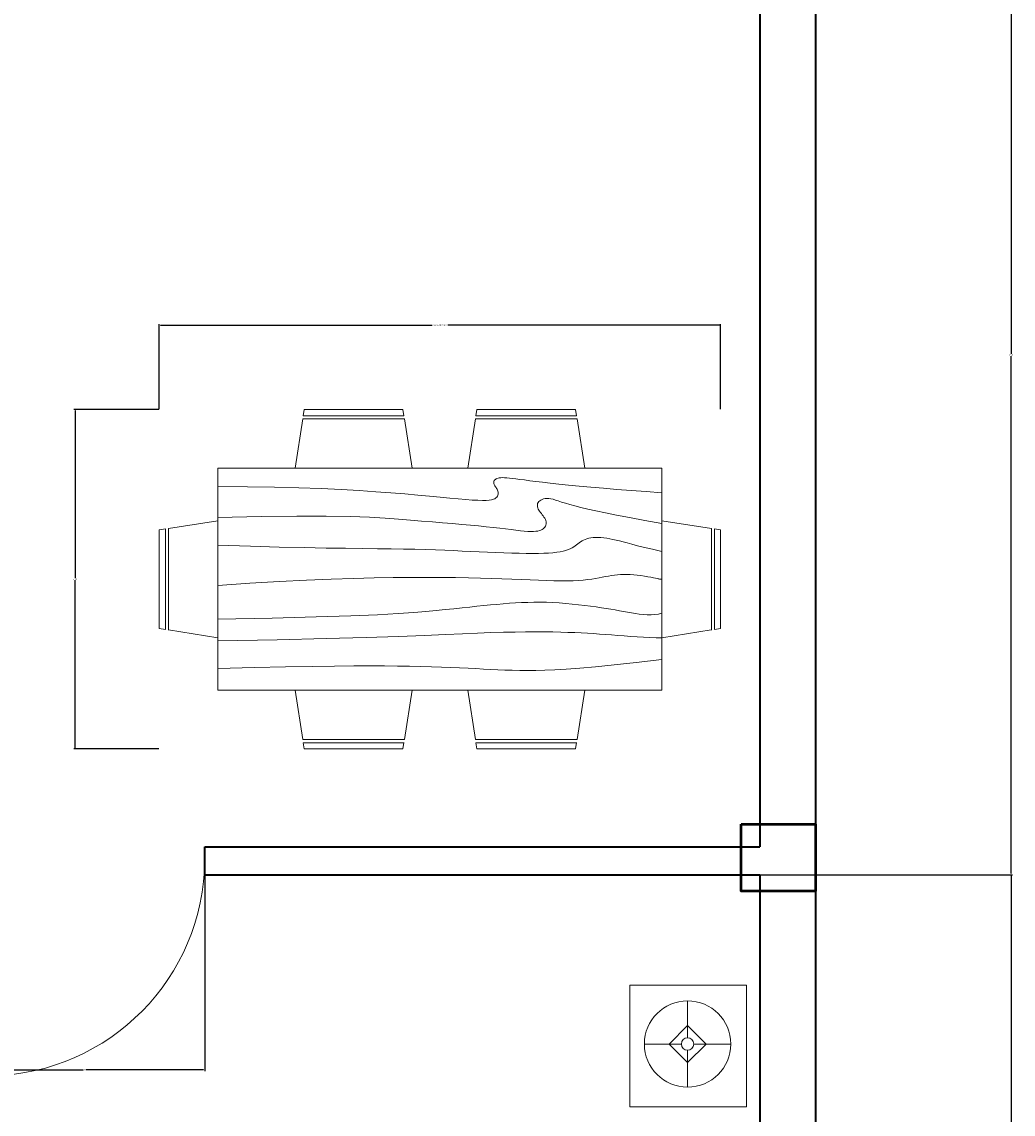
# Model space of a CAD drawing. Units: inches. Extents: x 50 to 2003, y -28 to 675.
# Tile 7 of 10: x 795 to 956, y 160 to 337. Entities that reach past the tile are written whole.
import ezdxf

# ---------------------------------------------------------------- set-up
doc = ezdxf.new("R2010")
doc.units = ezdxf.units.IN
for name, color, linetype, lineweight in [('A-ANNO-DIMS', 2, 'Continuous', 18), ('A-COLS', 1, 'Continuous', 50), ('A-DOOR', 4, 'Continuous', 18), ('A-FURN', 8, 'Continuous', 18), ('A-FURN-LITE', 9, 'Continuous', 13), ('A-WALL', 7, 'Continuous', 35)]:
    doc.layers.add(name, color=color, linetype=linetype, lineweight=lineweight)
doc.styles.get("Standard").update_dxf_attribs({"font": 'arial.ttf'})
doc.dimstyles.get("Standard").update_dxf_attribs({"dimtxt": 0.18, "dimasz": 0.18, "dimexe": 0.18, "dimexo": 0.0625, "dimgap": 0.09, "dimtad": 0, "dimtih": 1, "dimtoh": 1, "dimdec": 4, "dimzin": 0, "dimdsep": 46, "dimtxsty": 'Standard', "dimcen": 0.09, "dimadec": 0, "dimazin": 0, "dimtfac": 1, "dimtdec": 4, "dimtofl": 0, "dimtmove": 0, "dimatfit": 3, "dimfxl": 1, "dimtolj": 1, "dimtzin": 0, "dimarcsym": 0})

# ---------------------------------------------------------------- blocks, each defined once
blk = doc.blocks.new('Dining Set - 36 x 72 in.')
for p, q in [((-22, 27.5), (-22.1562, 26.50042)), ((-22, 27.5), (-6, 27.5)), ((-5.8437, 26.49966), (-6, 27.5)), ((6, 27.5), (5.8438, 26.50042)), ((6, 27.5), (22, 27.5)), ((22.1563, 26.49966), (22, 27.5)), ((-22.2343, 26.00059), (-23.4847, 17.99762)), ((-22.2304, 26), (-5.7608, 26)), ((-5.8416, 26.5), (-22.1534, 26.5)), ((-4.5152, 17.99762), (-5.7655, 25.99926)), ((5.7657, 26.00059), (4.5153, 17.99762)), ((5.7696, 26), (22.2392, 26)), ((22.1584, 26.5), (5.8466, 26.5)), ((23.4848, 17.99762), (22.2345, 25.99926)), ((36, 18), (-36, 18)), ((-36, 18), (-36, -18)), ((36, -18), (36, 18)), ((-44.0006, 8.23428), (-35.9976, 9.48474)), ((44.0006, 8.23428), (35.9976, 9.48474)), ((-45.5, 8), (-44.5004, 8.15617)), ((-45.5, 8), (-45.5, -8)), ((-44.5, -8.15843), (-44.5, 8.15338)), ((-44, 8.23041), (-44, -8.23915)), ((44, 8.23041), (44, -8.23915)), ((44.5, -8.15843), (44.5, 8.15338)), ((45.5, 8), (44.5005, 8.15617)), ((45.5, 8), (45.5, -8)), ((-44.4997, -8.15631), (-45.5, -8)), ((-35.9976, -9.48476), (-43.9993, -8.2345)), ((35.9976, -9.48476), (43.9993, -8.2345)), ((44.4997, -8.15631), (45.5, -8)), ((-36, -18), (36, -18)), ((-22.2343, -26.0006), (-23.4847, -17.99762)), ((-4.5152, -17.99762), (-5.7655, -25.99928)), ((5.7657, -26.0006), (4.5153, -17.99762)), ((23.4848, -17.99762), (22.2345, -25.99928)), ((-22.2304, -26), (-5.7608, -26)), ((-22, -27.5), (-22.1562, -26.50044)), ((-5.8416, -26.5), (-22.1534, -26.5)), ((-5.8437, -26.49967), (-6, -27.5)), ((5.7696, -26), (22.2392, -26)), ((6, -27.5), (5.8438, -26.50044)), ((22.1584, -26.5), (5.8466, -26.5)), ((22.1563, -26.49967), (22, -27.5)), ((-22, -27.5), (-6, -27.5)), ((6, -27.5), (22, -27.5))]:
    blk.add_line(p, q)
for points in [[(-36, 15), (-31.1772, 14.97754), (-26.8079, 14.91406), (-22.8538, 14.81543), (-19.276, 14.6875), (-16.0362, 14.53613), (-13.0957, 14.36718), (-10.4159, 14.18652), (-7.9583, 14), (-5.6904, 13.81315), (-3.6035, 13.63021), (-1.6954, 13.45508), (0.0365, 13.29166), (1.5945, 13.14388), (2.9811, 13.01562), (4.1988, 12.9108), (5.25, 12.83333), (6.1393, 12.78613), (6.8802, 12.76823), (7.4883, 12.77767), (7.9792, 12.8125), (8.3685, 12.87077), (8.6719, 12.95052), (8.9049, 13.0498), (9.0833, 13.16666), (9.2205, 13.29899), (9.3216, 13.44401), (9.3895, 13.59879), (9.4271, 13.76041), (9.4373, 13.92594), (9.4232, 14.09245), (9.3875, 14.257), (9.3333, 14.41666), (9.2638, 14.56917), (9.1836, 14.71484), (9.0975, 14.85465), (9.0104, 14.98958), (8.9272, 15.1206), (8.8529, 15.2487), (8.7922, 15.37483), (8.75, 15.5), (8.7305, 15.62467), (8.7344, 15.74739), (8.7617, 15.86621), (8.8125, 15.97916), (8.8867, 16.08431), (8.9844, 16.17968), (9.1055, 16.26334), (9.25, 16.33333), (9.4189, 16.38802), (9.6172, 16.42708), (9.8506, 16.45052), (10.125, 16.45833), (10.4463, 16.45052), (10.8203, 16.42708), (11.2529, 16.38802), (11.75, 16.33333), (12.3184, 16.26318), (12.9694, 16.17838), (13.7151, 16.07991), (14.5677, 15.96875), (15.5395, 15.84586), (16.6426, 15.71224), (17.8893, 15.56884), (19.2917, 15.41666), (20.859, 15.25667), (22.5879, 15.08984), (24.4721, 14.91715), (26.5052, 14.73958), (28.6809, 14.5581), (30.9929, 14.3737), (33.4347, 14.18733), (36, 14)], [(-36, 10), (-28.9766, 10.14274), (-23.1725, 10.20442), (-18.4241, 10.19775), (-14.5677, 10.13541), (-11.4399, 10.03011), (-8.877, 9.89453), (-6.7154, 9.74137), (-4.7917, 9.58333), (-2.9698, 9.43082), (-1.2246, 9.28515), (0.4415, 9.14534), (2.026, 9.01041), (3.5266, 8.87939), (4.9408, 8.7513), (6.266, 8.62516), (7.5, 8.5), (8.6411, 8.37549), (9.6914, 8.2539), (10.6538, 8.13818), (11.5312, 8.03125), (12.3267, 7.93603), (13.043, 7.85547), (13.6831, 7.79248), (14.25, 7.75), (14.7471, 7.7303), (15.1797, 7.73307), (15.5537, 7.75732), (15.875, 7.80208), (16.1494, 7.86637), (16.3828, 7.94922), (16.5811, 8.04964), (16.75, 8.16666), (16.8944, 8.29915), (17.0143, 8.44531), (17.1089, 8.60319), (17.1771, 8.77083), (17.218, 8.94629), (17.2305, 9.1276), (17.2137, 9.31282), (17.1667, 9.5), (17.0895, 9.6875), (16.987, 9.875), (16.8649, 10.0625), (16.7292, 10.25), (16.5856, 10.4375), (16.4401, 10.625), (16.2985, 10.8125), (16.1667, 11), (16.05, 11.18733), (15.9518, 11.3737), (15.8752, 11.5581), (15.8229, 11.73958), (15.798, 11.91715), (15.8034, 12.08984), (15.842, 12.25667), (15.9167, 12.41666), (16.0295, 12.56836), (16.1784, 12.70833), (16.3605, 12.83268), (16.5729, 12.9375), (16.8127, 13.01888), (17.0768, 13.07291), (17.3625, 13.0957), (17.6667, 13.08333), (17.9894, 13.03312), (18.3418, 12.94726), (18.7382, 12.82918), (19.1927, 12.68229), (19.7195, 12.51001), (20.3327, 12.31575), (21.0465, 12.10294), (21.875, 11.875), (22.8357, 11.63354), (23.959, 11.37304), (25.2786, 11.08618), (26.8282, 10.76562), (28.6414, 10.40405), (30.752, 9.99414), (33.1936, 9.52856), (36, 9)], [(-36, 5.5), (-30.7157, 5.3348), (-26.069, 5.20963), (-21.9946, 5.11767), (-18.4271, 5.05208), (-15.3009, 5.00602), (-12.5508, 4.97265), (-10.1112, 4.94515), (-7.9167, 4.91666), (-5.909, 4.88167), (-4.0586, 4.83984), (-2.3429, 4.79215), (-0.7396, 4.73958), (0.7739, 4.6831), (2.22, 4.6237), (3.6213, 4.56233), (5, 4.5), (6.373, 4.43782), (7.7344, 4.3776), (9.0723, 4.32129), (10.375, 4.27083), (11.6309, 4.22819), (12.8281, 4.19531), (13.9551, 4.17415), (15, 4.16666), (15.954, 4.17448), (16.819, 4.19791), (17.6001, 4.23698), (18.3021, 4.29166), (18.9299, 4.36198), (19.4883, 4.44791), (19.9823, 4.54948), (20.4167, 4.66666), (20.7969, 4.79899), (21.1302, 4.94401), (21.4245, 5.09879), (21.6875, 5.26041), (21.9271, 5.42594), (22.1511, 5.59245), (22.3672, 5.757), (22.5834, 5.91666), (22.8065, 6.06868), (23.0404, 6.21093), (23.2879, 6.34147), (23.5521, 6.45833), (23.8358, 6.55957), (24.142, 6.64323), (24.4735, 6.70735), (24.8334, 6.75), (25.2235, 6.76969), (25.642, 6.76692), (26.0858, 6.74267), (26.5521, 6.69791), (27.0379, 6.63362), (27.5404, 6.55078), (28.0565, 6.45036), (28.5834, 6.33333), (29.1242, 6.19987), (29.7071, 6.04687), (30.3661, 5.87044), (31.1354, 5.66666), (32.0493, 5.43164), (33.142, 5.16146), (34.4475, 4.85221), (36, 4.5)], [(-36, -1), (-30.7915, -0.6591), (-26.0195, -0.38216), (-21.6519, -0.16284), (-17.6563, 0.00521), (-14.0005, 0.12833), (-10.6523, 0.21289), (-7.5796, 0.26522), (-4.75, 0.29166), (-2.134, 0.29793), (0.2878, 0.28711), (2.5317, 0.26163), (4.6146, 0.22396), (6.5529, 0.17651), (8.3633, 0.12174), (10.0623, 0.06209), (11.6667, 0), (13.1899, -0.06201), (14.6341, -0.1211), (15.9982, -0.17432), (17.2813, -0.21875), (18.4823, -0.25147), (19.6003, -0.26953), (20.6343, -0.27002), (21.5834, -0.25), (22.4481, -0.20768), (23.2357, -0.14584), (23.9549, -0.06836), (24.6146, 0.02083), (25.2235, 0.11784), (25.7904, 0.21875), (26.3241, 0.31966), (26.8334, 0.41666), (27.3265, 0.50618), (27.8099, 0.58593), (28.2894, 0.65397), (28.7709, 0.70833), (29.2601, 0.74707), (29.763, 0.76823), (30.2855, 0.76985), (30.8334, 0.75), (31.4088, 0.70784), (31.9994, 0.64713), (32.589, 0.57275), (33.1615, 0.48958), (33.7008, 0.4025), (34.1908, 0.3164), (34.6153, 0.23616), (34.9584, 0.16666), (35.2099, 0.11165), (35.3848, 0.07031), (35.504, 0.04069), (35.5886, 0.02083), (35.6594, 0.00879), (35.7377, 0.0026), (35.8442, 0.00032), (36, 0)], [(-36, -6.5), (-27.1843, -6.31267), (-20.084, -6.1263), (-14.469, -5.9419), (-10.1094, -5.76042), (-6.7752, -5.58285), (-4.2363, -5.41016), (-2.2629, -5.24333), (-0.625, -5.08334), (0.8708, -4.93099), (2.2715, -4.78646), (3.5872, -4.64974), (4.8281, -4.52084), (6.0046, -4.39974), (7.127, -4.28646), (8.2053, -4.18099), (9.25, -4.08334), (10.2705, -3.99382), (11.2734, -3.91407), (12.2647, -3.84603), (13.25, -3.79167), (14.2354, -3.75293), (15.2266, -3.73177), (16.2295, -3.73015), (17.25, -3.75), (18.2912, -3.79248), (19.3451, -3.85547), (20.4009, -3.93604), (21.4479, -4.03125), (22.4754, -4.13819), (23.4727, -4.25391), (24.4289, -4.37549), (25.3334, -4.5), (26.1785, -4.62492), (26.9694, -4.74935), (27.7145, -4.87281), (28.4219, -4.99479), (29.1, -5.11483), (29.7572, -5.23242), (30.4016, -5.34709), (31.0417, -5.45834), (31.6837, -5.56437), (32.3262, -5.65821), (32.9658, -5.73153), (33.599, -5.77604), (34.2224, -5.78345), (34.8327, -5.74545), (35.4264, -5.65373), (36, -5.5)], [(-36, -10), (-26.4022, -9.81299), (-18.4675, -9.62891), (-11.9839, -9.45069), (-6.7396, -9.28125), (-2.5226, -9.12354), (0.8789, -8.98047), (3.6769, -8.85498), (6.0833, -8.75), (8.2767, -8.66765), (10.3021, -8.60677), (12.1712, -8.56543), (13.8958, -8.54167), (15.4876, -8.53353), (16.9583, -8.53907), (18.3197, -8.55632), (19.5834, -8.58334), (20.7616, -8.61841), (21.8685, -8.66081), (22.9188, -8.71004), (23.9271, -8.76563), (24.9081, -8.82707), (25.8763, -8.89388), (26.8465, -8.96558), (27.8334, -9.04167), (28.8474, -9.12118), (29.8828, -9.20117), (30.93, -9.27824), (31.9792, -9.34896), (33.0205, -9.40991), (34.0443, -9.45768), (35.0407, -9.48885), (36, -9.5)], [(-36, -14.5), (-30.0881, -14.33513), (-25.0332, -14.21224), (-20.7312, -14.12647), (-17.0781, -14.07292), (-13.97, -14.04671), (-11.3027, -14.04297), (-8.9724, -14.05681), (-6.875, -14.08334), (-4.9224, -14.11833), (-3.0905, -14.16016), (-1.3709, -14.20785), (0.2448, -14.26042), (1.7647, -14.3169), (3.1973, -14.3763), (4.5507, -14.43767), (5.8333, -14.5), (7.0554, -14.5621), (8.235, -14.62175), (9.3922, -14.67652), (10.5469, -14.72396), (11.7192, -14.76164), (12.929, -14.78711), (14.1965, -14.79794), (15.5417, -14.79167), (16.9933, -14.76424), (18.6152, -14.70508), (20.4804, -14.60197), (22.6615, -14.44271), (25.2312, -14.21509), (28.2624, -13.9069), (31.8277, -13.50594), (36, -13)]]:
    blk.add_lwpolyline(points)
blk = doc.blocks.new('Lamp - Table')
for p, q in [((0, 7), (0, 1)), ((0, 3), (-3, 0)), ((3, 0), (0, 3)), ((-1, 0), (-7, 0)), ((-3, 0), (0, -3)), ((0, -3), (3, 0)), ((1, 0), (7, 0)), ((0, -1), (0, -7))]:
    blk.add_line(p, q)
for radius in [7, 1]:
    blk.add_circle((0, 0), radius)
blk = doc.blocks.new('NIGHTSTAND-COMPACT')
blk.add_lwpolyline([(0, 19.73), (0, 0), (18.92, 0), (18.92, 19.73)], close=True)
blk = doc.blocks.new('*D41')
at = {"layer": 'A-ANNO-DIMS', "color": 0, "lineweight": -2, "transparency": 16777216}
for p, q in [((817.26, 274.59), (817.26, 288.36)), ((817.44, 288.18), (861.48, 288.18)), ((908.08, 288.18), (864.03, 288.18)), ((908.26, 274.59), (908.26, 288.36))]:
    blk.add_line(p, q, dxfattribs=at)
at = {"layer": 'A-ANNO-DIMS', "color": 0, "transparency": 16777216}
for points in [[(817.44, 288.21), (817.44, 288.15), (817.26, 288.18)], [(908.08, 288.21), (908.08, 288.15), (908.26, 288.18)]]:
    blk.add_solid(points, dxfattribs=at)
at = {"layer": 'Defpoints', "color": 0, "transparency": 16777216}
for p in [(908.26, 288.18), (817.26, 274.53), (908.26, 274.53)]:
    blk.add_point(p, dxfattribs=at)
at = {"layer": 'A-ANNO-DIMS', "color": 0, "transparency": 16777216, "insert": (862.76, 288.18), "char_height": 0.18, "attachment_point": 5}
blk.add_mtext('\\A1;DINING SET 91 TYP.', dxfattribs=at)
blk = doc.blocks.new('*D42')
at = {"layer": 'A-ANNO-DIMS', "color": 0, "lineweight": -2, "transparency": 16777216}
for p, q in [((817.19, 274.53), (803.43, 274.53)), ((803.61, 274.35), (803.61, 247.21)), ((803.61, 219.71), (803.61, 246.84)), ((817.19, 219.53), (803.43, 219.53))]:
    blk.add_line(p, q, dxfattribs=at)
at = {"layer": 'A-ANNO-DIMS', "color": 0, "transparency": 16777216}
for points in [[(803.58, 274.35), (803.64, 274.35), (803.61, 274.53)], [(803.58, 219.71), (803.64, 219.71), (803.61, 219.53)]]:
    blk.add_solid(points, dxfattribs=at)
at = {"layer": 'Defpoints', "color": 0, "transparency": 16777216}
for p in [(803.61, 274.53), (817.26, 274.53), (817.26, 219.53)]:
    blk.add_point(p, dxfattribs=at)
at = {"layer": 'A-ANNO-DIMS', "color": 0, "transparency": 16777216, "insert": (803.61, 247.03), "char_height": 0.18, "attachment_point": 5}
blk.add_mtext('\\A1;55 TYP.', dxfattribs=at)
blk = doc.blocks.new('*D81')
at = {"layer": 'A-ANNO-DIMS', "color": 0, "lineweight": -2, "transparency": 16777216}
for p, q in [((914.68, 199.12), (955.56, 199.12)), ((955.38, 198.94), (955.38, 125.05)), ((955.38, 50.8), (955.38, 124.69)), ((914.68, 50.62), (955.56, 50.62))]:
    blk.add_line(p, q, dxfattribs=at)
at = {"layer": 'A-ANNO-DIMS', "color": 0, "transparency": 16777216}
for points in [[(955.35, 198.94), (955.41, 198.94), (955.38, 199.12)], [(955.35, 50.8), (955.41, 50.8), (955.38, 50.62)]]:
    blk.add_solid(points, dxfattribs=at)
at = {"layer": 'Defpoints', "color": 0, "transparency": 16777216}
for p in [(914.62, 199.12), (955.38, 199.12), (914.62, 50.62)]:
    blk.add_point(p, dxfattribs=at)
at = {"layer": 'A-ANNO-DIMS', "color": 0, "transparency": 16777216, "insert": (955.38, 124.87), "char_height": 0.18, "attachment_point": 5}
blk.add_mtext('\\A1;148.5', dxfattribs=at)
blk = doc.blocks.new('*D82')
at = {"layer": 'A-ANNO-DIMS', "color": 0, "lineweight": -2, "transparency": 16777216}
for p, q in [((914.68, 367.62), (955.56, 367.62)), ((955.38, 367.44), (955.38, 283.55)), ((955.38, 199.3), (955.38, 283.19)), ((914.68, 199.12), (955.56, 199.12))]:
    blk.add_line(p, q, dxfattribs=at)
at = {"layer": 'A-ANNO-DIMS', "color": 0, "transparency": 16777216}
for points in [[(955.35, 367.44), (955.41, 367.44), (955.38, 367.62)], [(955.35, 199.3), (955.41, 199.3), (955.38, 199.12)]]:
    blk.add_solid(points, dxfattribs=at)
at = {"layer": 'Defpoints', "color": 0, "transparency": 16777216}
for p in [(914.62, 367.62), (955.38, 367.62), (914.62, 199.12)]:
    blk.add_point(p, dxfattribs=at)
at = {"layer": 'A-ANNO-DIMS', "color": 0, "transparency": 16777216, "insert": (955.38, 283.37), "char_height": 0.18, "attachment_point": 5}
blk.add_mtext('\\A1;168.5', dxfattribs=at)
blk = doc.blocks.new('*D94')
at = {"layer": 'A-ANNO-DIMS', "color": 0, "lineweight": -2, "transparency": 16777216}
for p, q in [((785.62, 199.06), (785.62, 167.29)), ((824.62, 199.06), (824.62, 167.29)), ((785.8, 167.47), (804.9, 167.47)), ((824.44, 167.47), (805.34, 167.47))]:
    blk.add_line(p, q, dxfattribs=at)
at = {"layer": 'A-ANNO-DIMS', "color": 0, "transparency": 16777216}
for points in [[(785.8, 167.5), (785.8, 167.44), (785.62, 167.47)], [(824.44, 167.5), (824.44, 167.44), (824.62, 167.47)]]:
    blk.add_solid(points, dxfattribs=at)
at = {"layer": 'Defpoints', "color": 0, "transparency": 16777216}
for p in [(785.62, 199.12), (824.62, 199.12), (785.62, 167.47)]:
    blk.add_point(p, dxfattribs=at)
at = {"layer": 'A-ANNO-DIMS', "color": 0, "transparency": 16777216, "insert": (805.12, 167.47), "char_height": 0.18, "attachment_point": 5}
blk.add_mtext('\\A1;39', dxfattribs=at)

msp = doc.modelspace()

# ---------------------------------------------------------------- linework, layer by layer
at = {"layer": 'A-COLS'}
msp.add_lwpolyline([(911.5683, 207.3037), (923.6383, 207.3037), (923.6383, 196.4326), (911.5683, 196.4326)], close=True, dxfattribs=at)
at = {"layer": 'A-DOOR'}
msp.add_arc((789.3225, 201.8282), 35.3264, 268.663025, 356.673823, dxfattribs=at)
at = {"layer": 'A-WALL'}
for p, q in [((923.6163, 618.6217), (923.6163, 3.6217)), ((914.6163, 367.6216), (914.6163, 203.6217)), ((824.6163, 199.1216), (824.6163, 203.6217)), ((824.6163, 203.6217), (914.6163, 203.6217)), ((824.6163, 199.1216), (914.6163, 199.1216)), ((914.6163, 199.1216), (914.6163, 55.1217))]:
    msp.add_line(p, q, dxfattribs=at)

# ---------------------------------------------------------------- block references
at = {"layer": 'A-FURN'}
msp.add_blockref('Dining Set - 36 x 72 in.', (862.7552, 247.0251), dxfattribs=at)
at = {"layer": 'A-FURN', "rotation": 180}
msp.add_blockref('NIGHTSTAND-COMPACT', (912.4473, 181.2329), dxfattribs=at)
at = {"layer": 'A-FURN-LITE', "rotation": 270}
msp.add_blockref('Lamp - Table', (902.8991, 171.6786), dxfattribs=at)

# ---------------------------------------------------------------- dimensions: what is measured, and where the dimension line sits
at = {"layer": 'A-ANNO-DIMS'}
for base, p1, p2, angle, override, picture, middle in [((955.3793, 367.6216), (914.6163, 199.1216), (914.6163, 367.6216), 90, {"dimdec": 1, "dimlfac": 1, "dimrnd": 0, "dimzin": 0, "dimdsep": 46, "dimlunit": 2}, '*D82', (955.3793, 283.3716)), ((785.6163, 167.4717), (824.6163, 199.1216), (785.6163, 199.1216), 180, {"dimdec": 0, "dimlfac": 1, "dimrnd": 0, "dimzin": 0, "dimdsep": 46, "dimlunit": 2}, '*D94', (805.1163, 167.4717)), ((955.3793, 199.1216), (914.6163, 50.6217), (914.6163, 199.1216), 90, {"dimdec": 1, "dimlfac": 1, "dimrnd": 0, "dimzin": 0, "dimdsep": 46, "dimlunit": 2}, '*D81', (955.3793, 124.8716))]:
    dim = msp.add_linear_dim(base=base, p1=p1, p2=p2, angle=angle, dimstyle='Standard', override=override, dxfattribs=at)
    dim.commit()
    dim.dimension.update_dxf_attribs({"geometry": picture, "text_midpoint": middle})
dim = msp.add_linear_dim(base=(908.2552, 288.1751), p1=(817.2552, 274.5251), p2=(908.2552, 274.5251), text='DINING SET <> TYP.', dimstyle='Standard', override={"dimdec": 0, "dimlfac": 1, "dimrnd": 0, "dimzin": 0, "dimdsep": 46, "dimlunit": 2}, dxfattribs=at)
dim.commit()
dim.dimension.update_dxf_attribs({"geometry": '*D41', "text_midpoint": (862.7552, 288.1751)})
dim = msp.add_linear_dim(base=(803.6052, 274.5251), p1=(817.2552, 219.5251), p2=(817.2552, 274.5251), angle=90, text='<> TYP.', dimstyle='Standard', override={"dimdec": 0, "dimlfac": 1, "dimrnd": 0, "dimzin": 0, "dimdsep": 46, "dimlunit": 2}, dxfattribs=at)
dim.commit()
dim.dimension.update_dxf_attribs({"geometry": '*D42', "text_midpoint": (803.6052, 247.0251)})

doc.saveas('drawing.dxf')
